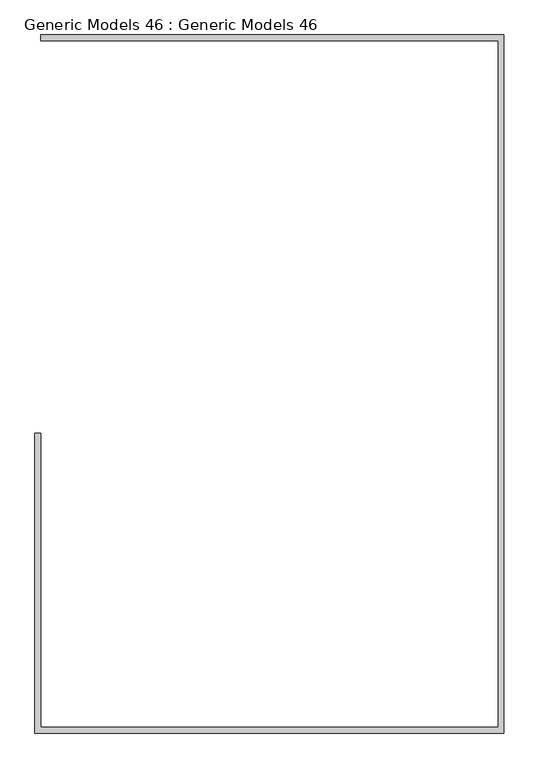
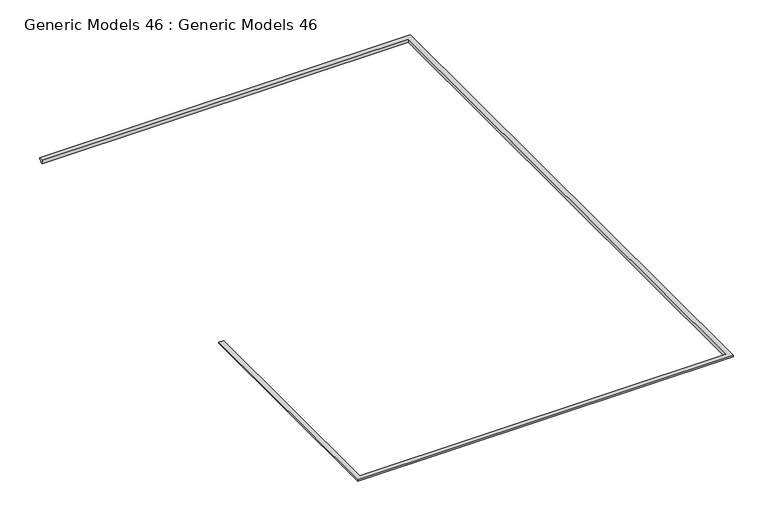
"""IFC4 building model written with IfcOpenShell, lengths in millimetres: proxy geometry, Generic Models 46 : Generic Models 46."""

from ifc_helpers import new_model, si_unit, origin, place, context, project, spatial, faceted_brep, source, transform, mapped, element, save


def generic_models_46_generic_models_46_dc31fbd0(model_context):
    return source(origin(), model_context, "Body", "Brep", [
        faceted_brep([(-6432.5887202, 13410.9309003, 18897.6), (-6432.5887202, 13410.9309003, 18853.15), (-6432.5887202, 13360.1309003, 18853.15), (-6432.5887202, 13360.1309003, 18821.4), (-6432.5887202, 13315.6809003, 18821.4), (-6432.5887202, 13315.6809003, 18796.0), (-6432.5887202, 13271.2309003, 18796.0), (-6432.5887202, 13271.2309003, 18897.6), (-6572.2887202, 3835.1309003, 18897.6), (-6432.5887202, 3835.1309003, 18897.6), (-6432.5887202, 3835.1309003, 18796.0), (-6477.0387202, 3835.1309003, 18796.0), (-6477.0387202, 3835.1309003, 18821.4), (-6521.4887202, 3835.1309003, 18821.4), (-6521.4887202, 3835.1309003, 18853.15), (-6572.2887202, 3835.1309003, 18853.15), (4706.8987798, 13410.9309003, 18897.6), (4706.8987798, 13410.9309003, 18853.15), (4706.8987798, -3378.4690997, 18853.15), (-6572.2887202, -3378.4690997, 18853.15), (-6521.4887202, -3327.6690997, 18853.15), (4656.0987798, -3327.6690997, 18853.15), (4656.0987798, 13360.1309003, 18853.15), (4656.0987798, 13360.1309003, 18821.4), (4656.0987798, -3327.6690997, 18821.4), (-6521.4887202, -3327.6690997, 18821.4), (-6477.0387202, -3283.2190997, 18821.4), (4611.6487798, -3283.2190997, 18821.4), (4611.6487798, 13315.6809003, 18821.4), (4611.6487798, 13315.6809003, 18796.0), (4611.6487798, -3283.2190997, 18796.0), (-6477.0387202, -3283.2190997, 18796.0), (-6432.5887202, -3238.7690997, 18796.0), (4567.1987798, -3238.7690997, 18796.0), (4567.1987798, 13271.2309003, 18796.0), (4567.1987798, 13271.2309003, 18897.6), (4567.1987798, -3238.7690997, 18897.6), (-6432.5887202, -3238.7690997, 18897.6), (-6572.2887202, -3378.4690997, 18897.6), (4706.8987798, -3378.4690997, 18897.6)], [[[0, 1, 2, 3, 4, 5, 6, 7]], [[8, 9, 10, 11, 12, 13, 14, 15]], [[1, 0, 16, 17]], [[2, 1, 17, 18, 19, 15, 14, 20, 21, 22]], [[3, 2, 22, 23]], [[4, 3, 23, 24, 25, 13, 12, 26, 27, 28]], [[5, 4, 28, 29]], [[6, 5, 29, 30, 31, 11, 10, 32, 33, 34]], [[7, 6, 34, 35]], [[0, 7, 35, 36, 37, 9, 8, 38, 39, 16]], [[17, 16, 39, 18]], [[23, 22, 21, 24]], [[29, 28, 27, 30]], [[35, 34, 33, 36]], [[18, 39, 38, 19]], [[24, 21, 20, 25]], [[30, 27, 26, 31]], [[36, 33, 32, 37]], [[19, 38, 8, 15]], [[25, 20, 14, 13]], [[31, 26, 12, 11]], [[37, 32, 10, 9]]]),
    ])


if __name__ == "__main__":
    model = new_model("IFC4")
    model_context = context("Model", 3, world=origin())
    ifc_project = project(units=[si_unit("LENGTHUNIT", "METRE", prefix="MILLI")], contexts=[model_context])
    site = spatial("IfcSite", under=ifc_project)
    building = spatial("IfcBuilding", under=site)
    placement = place(None, origin())
    generic_models_46_generic_models_46_shape = generic_models_46_generic_models_46_dc31fbd0(model_context)
    element("IfcBuildingElementProxy", 1, Name="Generic Models 46 : Generic Models 46", ObjectType="Generic Models 46 : Generic Models 46", at=placement, inside=building, context=model_context, shape_type="MappedRepresentation", body=[
        mapped(generic_models_46_generic_models_46_shape, transform((0.0, 0.0, 0.0), x_axis=(1.0, 0.0, 0.0), y_axis=(0.0, 1.0, 0.0), z_axis=(0.0, 0.0, 1.0))),
    ])
    save(model, "model.ifc")

# Revit data of these elements
# Element 1 (IfcBuildingElementProxy, "Generic Models 46 : Generic Models 46")
#   Materials on its faces: "white"
# Materials
#   "white": class "Generic", colour RGB 120 120 120, transparency 0, Cost = 0
